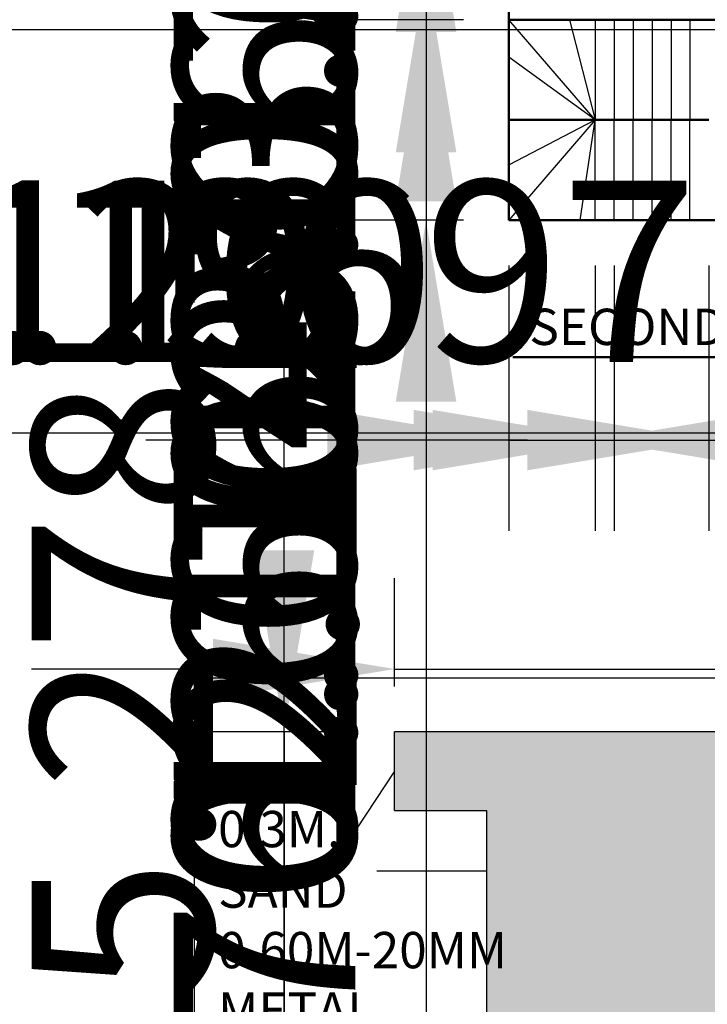
# Model space of a CAD drawing. Units: metres. Extents: x 782 to 1487, y 1262 to 7446.
# Tile 8 of 25: x 821.23 to 830.69, y 1279.51 to 1293.07. Entities that reach past the tile are written whole.
import ezdxf

# ---------------------------------------------------------------- set-up
doc = ezdxf.new("R2010")
doc.units = ezdxf.units.M
for name, color, linetype, lineweight in [('A-ANNO-DIMS', 2, 'Continuous', 18), ('A-ANNO-TEXT', 3, 'Continuous', 18), ('A-DETL', 7, 'Continuous', 25), ('A-DETL-PATT', 9, 'Continuous', 13), ('A-FLOR-STRS', 3, 'Continuous', 25), ('A-WALL', 7, 'Continuous', 50)]:
    doc.layers.add(name, color=color, linetype=linetype, lineweight=lineweight)
doc.styles.get("Standard").update_dxf_attribs({"font": 'arial.ttf'})
doc.dimstyles.new('ISO-25', dxfattribs={"dimtxt": 2.5, "dimasz": 2.5, "dimexe": 1.25, "dimexo": 0.625, "dimtad": 1, "dimtxsty": 'Standard', "dimcen": 2.5, "dimadec": 0, "dimazin": 0, "dimtfac": 1, "dimtmove": 0, "dimatfit": 3, "dimfxl": 1, "dimarcsym": 0})

# ---------------------------------------------------------------- blocks, each defined once
blk = doc.blocks.new('*D10')
at = {"layer": 'A-ANNO-DIMS', "color": 0, "lineweight": -2, "transparency": 16777216}
for p, q in [((825.73, 1277.527), (825.73, 1276.166)), ((826.753, 1277.552), (826.753, 1276.166)), ((823.23, 1277.416), (820.73, 1277.416)), ((825.73, 1277.416), (826.753, 1277.416)), ((829.253, 1277.416), (839.235, 1277.416))]:
    blk.add_line(p, q, dxfattribs=at)
at = {"layer": 'A-ANNO-DIMS', "color": 0, "transparency": 16777216}
for points in [[(823.23, 1277.833), (823.23, 1276.999), (825.73, 1277.416)], [(829.253, 1277.833), (829.253, 1276.999), (826.753, 1277.416)]]:
    blk.add_solid(points, dxfattribs=at)
at = {"layer": 'Defpoints', "color": 0, "transparency": 16777216}
for p in [(826.753, 1278.177), (825.73, 1278.152), (826.753, 1277.416)]:
    blk.add_point(p, dxfattribs=at)
at = {"layer": 'A-ANNO-DIMS', "color": 0, "transparency": 16777216, "insert": (835.494, 1279.543), "char_height": 2.5, "attachment_point": 5}
blk.add_mtext('1,02', dxfattribs=at)
blk = doc.blocks.new('*D22')
at = {"layer": 'A-ANNO-DIMS', "color": 0, "lineweight": -2, "transparency": 16777216}
for p, q in [((812.79, 1292.934), (810.29, 1292.934)), ((815.29, 1292.934), (816.179, 1292.934)), ((818.679, 1292.934), (848.834, 1292.934)), ((815.29, 1292.442), (815.29, 1291.684)), ((816.179, 1292.442), (816.179, 1291.684))]:
    blk.add_line(p, q, dxfattribs=at)
at = {"layer": 'A-ANNO-DIMS', "color": 0, "transparency": 16777216}
for points in [[(812.79, 1293.351), (812.79, 1292.517), (815.29, 1292.934)], [(818.679, 1293.351), (818.679, 1292.517), (816.179, 1292.934)]]:
    blk.add_solid(points, dxfattribs=at)
at = {"layer": 'Defpoints', "color": 0, "transparency": 16777216}
for p in [(815.29, 1293.067), (816.179, 1293.067), (816.179, 1292.934)]:
    blk.add_point(p, dxfattribs=at)
at = {"layer": 'A-ANNO-DIMS', "color": 0, "transparency": 16777216, "insert": (835.007, 1294.852), "char_height": 2.5, "attachment_point": 5}
blk.add_mtext('DOOR 0.89 TYP.', dxfattribs=at)
blk = doc.blocks.new('*D24')
at = {"layer": 'A-ANNO-DIMS', "color": 0, "lineweight": -2, "transparency": 16777216}
for p, q in [((811.209, 1294.423), (808.709, 1294.423)), ((813.709, 1294.423), (814.559, 1294.423)), ((817.059, 1294.423), (852.649, 1294.423)), ((813.709, 1293.926), (813.709, 1293.173)), ((814.559, 1293.926), (814.559, 1293.173))]:
    blk.add_line(p, q, dxfattribs=at)
at = {"layer": 'A-ANNO-DIMS', "color": 0, "transparency": 16777216}
for points in [[(811.209, 1294.84), (811.209, 1294.006), (813.709, 1294.423)], [(817.059, 1294.84), (817.059, 1294.006), (814.559, 1294.423)]]:
    blk.add_solid(points, dxfattribs=at)
at = {"layer": 'Defpoints', "color": 0, "transparency": 16777216}
for p in [(813.709, 1294.551), (814.559, 1294.551), (814.559, 1294.423)]:
    blk.add_point(p, dxfattribs=at)
at = {"layer": 'A-ANNO-DIMS', "color": 0, "transparency": 16777216, "insert": (836.104, 1296.342), "char_height": 2.5, "attachment_point": 5}
blk.add_mtext('DOOR D2 0.85 TYP.', dxfattribs=at)
blk = doc.blocks.new('*D73')
at = {"layer": 'A-ANNO-DIMS', "color": 0, "lineweight": -2, "transparency": 16777216}
for p, q in [((812.13, 1289.68), (812.13, 1286.127)), ((813.319, 1289.68), (813.319, 1286.127)), ((809.63, 1287.377), (807.13, 1287.377)), ((812.13, 1287.377), (813.319, 1287.377)), ((815.819, 1287.377), (825.832, 1287.377))]:
    blk.add_line(p, q, dxfattribs=at)
at = {"layer": 'A-ANNO-DIMS', "color": 0, "transparency": 16777216}
for points in [[(809.63, 1287.794), (809.63, 1286.96), (812.13, 1287.377)], [(815.819, 1287.794), (815.819, 1286.96), (813.319, 1287.377)]]:
    blk.add_solid(points, dxfattribs=at)
at = {"layer": 'Defpoints', "color": 0, "transparency": 16777216}
for p in [(812.13, 1290.305), (813.319, 1290.305), (813.319, 1287.377)]:
    blk.add_point(p, dxfattribs=at)
at = {"layer": 'A-ANNO-DIMS', "color": 0, "transparency": 16777216, "insert": (822.076, 1289.278), "char_height": 2.5, "attachment_point": 5}
blk.add_mtext('1.19', dxfattribs=at)
blk = doc.blocks.new('*D74')
at = {"layer": 'A-ANNO-DIMS', "color": 0, "lineweight": -2, "transparency": 16777216}
for p, q in [((813.319, 1289.68), (813.319, 1286.127)), ((813.58, 1289.68), (813.58, 1286.127)), ((810.819, 1287.377), (808.319, 1287.377)), ((813.319, 1287.377), (813.58, 1287.377)), ((816.08, 1287.377), (826.322, 1287.377))]:
    blk.add_line(p, q, dxfattribs=at)
at = {"layer": 'A-ANNO-DIMS', "color": 0, "transparency": 16777216}
for points in [[(810.819, 1287.794), (810.819, 1286.96), (813.319, 1287.377)], [(816.08, 1287.794), (816.08, 1286.96), (813.58, 1287.377)]]:
    blk.add_solid(points, dxfattribs=at)
at = {"layer": 'Defpoints', "color": 0, "transparency": 16777216}
for p in [(813.319, 1290.305), (813.58, 1290.305), (813.58, 1287.377)]:
    blk.add_point(p, dxfattribs=at)
at = {"layer": 'A-ANNO-DIMS', "color": 0, "transparency": 16777216, "insert": (822.451, 1289.278), "char_height": 2.5, "attachment_point": 5}
blk.add_mtext('0.26', dxfattribs=at)
blk = doc.blocks.new('*D75')
at = {"layer": 'A-ANNO-DIMS', "color": 0, "lineweight": -2, "transparency": 16777216}
for p, q in [((813.58, 1289.68), (813.58, 1286.127)), ((814.883, 1289.68), (814.883, 1286.127)), ((811.08, 1287.377), (808.58, 1287.377)), ((813.58, 1287.377), (814.883, 1287.377)), ((817.383, 1287.377), (827.383, 1287.377))]:
    blk.add_line(p, q, dxfattribs=at)
at = {"layer": 'A-ANNO-DIMS', "color": 0, "transparency": 16777216}
for points in [[(811.08, 1287.794), (811.08, 1286.96), (813.58, 1287.377)], [(817.383, 1287.794), (817.383, 1286.96), (814.883, 1287.377)]]:
    blk.add_solid(points, dxfattribs=at)
at = {"layer": 'Defpoints', "color": 0, "transparency": 16777216}
for p in [(813.58, 1290.305), (814.883, 1290.305), (814.883, 1287.377)]:
    blk.add_point(p, dxfattribs=at)
at = {"layer": 'A-ANNO-DIMS', "color": 0, "transparency": 16777216, "insert": (823.633, 1289.279), "char_height": 2.5, "attachment_point": 5}
blk.add_mtext('1.30', dxfattribs=at)
blk = doc.blocks.new('*D76')
at = {"layer": 'A-ANNO-DIMS', "color": 0, "lineweight": -2, "transparency": 16777216}
for p, q in [((814.883, 1289.68), (814.883, 1286.127)), ((816.58, 1289.68), (816.58, 1286.127)), ((812.383, 1287.377), (809.883, 1287.377)), ((814.883, 1287.377), (816.58, 1287.377)), ((819.08, 1287.377), (831.031, 1287.377))]:
    blk.add_line(p, q, dxfattribs=at)
at = {"layer": 'A-ANNO-DIMS', "color": 0, "transparency": 16777216}
for points in [[(812.383, 1287.794), (812.383, 1286.96), (814.883, 1287.377)], [(819.08, 1287.794), (819.08, 1286.96), (816.58, 1287.377)]]:
    blk.add_solid(points, dxfattribs=at)
at = {"layer": 'Defpoints', "color": 0, "transparency": 16777216}
for p in [(814.883, 1290.305), (816.58, 1290.305), (816.58, 1287.377)]:
    blk.add_point(p, dxfattribs=at)
at = {"layer": 'A-ANNO-DIMS', "color": 0, "transparency": 16777216, "insert": (826.305, 1289.278), "char_height": 2.5, "attachment_point": 5}
blk.add_mtext('1.697', dxfattribs=at)
blk = doc.blocks.new('*D77')
at = {"layer": 'A-ANNO-DIMS', "color": 0, "lineweight": -2, "transparency": 16777216}
for p, q in [((826.821, 1309.827), (826.821, 1312.327)), ((827.337, 1307.327), (825.571, 1307.327)), ((826.821, 1307.327), (826.821, 1304.697)), ((827.567, 1304.697), (825.571, 1304.697)), ((826.821, 1302.197), (826.821, 1291.911))]:
    blk.add_line(p, q, dxfattribs=at)
at = {"layer": 'A-ANNO-DIMS', "color": 0, "transparency": 16777216}
for points in [[(826.404, 1309.827), (827.238, 1309.827), (826.821, 1307.327)], [(826.404, 1302.197), (827.238, 1302.197), (826.821, 1304.697)]]:
    blk.add_solid(points, dxfattribs=at)
at = {"layer": 'Defpoints', "color": 0, "transparency": 16777216}
for p in [(827.962, 1307.327), (826.821, 1304.697), (828.192, 1304.697)]:
    blk.add_point(p, dxfattribs=at)
at = {"layer": 'A-ANNO-DIMS', "color": 0, "transparency": 16777216, "insert": (824.919, 1295.804), "char_height": 2.5, "attachment_point": 5, "rotation": 90}
blk.add_mtext('2.63', dxfattribs=at)
blk = doc.blocks.new('*D78')
at = {"layer": 'A-ANNO-DIMS', "color": 0, "lineweight": -2, "transparency": 16777216}
for p, q in [((826.821, 1307.197), (826.821, 1309.697)), ((827.567, 1304.697), (825.571, 1304.697)), ((826.821, 1304.697), (826.821, 1302.822)), ((827.336, 1302.822), (825.571, 1302.822)), ((826.821, 1300.322), (826.821, 1290.308))]:
    blk.add_line(p, q, dxfattribs=at)
at = {"layer": 'A-ANNO-DIMS', "color": 0, "transparency": 16777216}
for points in [[(826.404, 1307.197), (827.238, 1307.197), (826.821, 1304.697)], [(826.404, 1300.322), (827.238, 1300.322), (826.821, 1302.822)]]:
    blk.add_solid(points, dxfattribs=at)
at = {"layer": 'Defpoints', "color": 0, "transparency": 16777216}
for p in [(828.192, 1304.697), (826.821, 1302.822), (827.961, 1302.822)]:
    blk.add_point(p, dxfattribs=at)
at = {"layer": 'A-ANNO-DIMS', "color": 0, "transparency": 16777216, "insert": (824.919, 1294.065), "char_height": 2.5, "attachment_point": 5, "rotation": 90}
blk.add_mtext('1.88', dxfattribs=at)
blk = doc.blocks.new('*D79')
at = {"layer": 'A-ANNO-DIMS', "color": 0, "lineweight": -2, "transparency": 16777216}
for p, q in [((826.821, 1305.322), (826.821, 1307.822)), ((827.336, 1302.822), (825.571, 1302.822)), ((826.821, 1302.822), (826.821, 1302.177)), ((827.567, 1302.177), (825.571, 1302.177)), ((826.821, 1299.677), (826.821, 1289.444))]:
    blk.add_line(p, q, dxfattribs=at)
at = {"layer": 'A-ANNO-DIMS', "color": 0, "transparency": 16777216}
for points in [[(826.404, 1305.322), (827.238, 1305.322), (826.821, 1302.822)], [(826.404, 1299.677), (827.238, 1299.677), (826.821, 1302.177)]]:
    blk.add_solid(points, dxfattribs=at)
at = {"layer": 'Defpoints', "color": 0, "transparency": 16777216}
for p in [(827.961, 1302.822), (826.821, 1302.177), (828.192, 1302.177)]:
    blk.add_point(p, dxfattribs=at)
at = {"layer": 'A-ANNO-DIMS', "color": 0, "transparency": 16777216, "insert": (824.919, 1293.311), "char_height": 2.5, "attachment_point": 5, "rotation": 90}
blk.add_mtext('0.64', dxfattribs=at)
blk = doc.blocks.new('*D80')
at = {"layer": 'A-ANNO-DIMS', "color": 0, "lineweight": -2, "transparency": 16777216}
for p, q in [((826.821, 1304.677), (826.821, 1307.177)), ((827.567, 1302.177), (825.571, 1302.177)), ((826.821, 1302.177), (826.821, 1299.809)), ((827.338, 1299.809), (825.571, 1299.809)), ((826.821, 1297.309), (826.821, 1287.022))]:
    blk.add_line(p, q, dxfattribs=at)
at = {"layer": 'A-ANNO-DIMS', "color": 0, "transparency": 16777216}
for points in [[(826.404, 1304.677), (827.238, 1304.677), (826.821, 1302.177)], [(826.404, 1297.309), (827.238, 1297.309), (826.821, 1299.809)]]:
    blk.add_solid(points, dxfattribs=at)
at = {"layer": 'Defpoints', "color": 0, "transparency": 16777216}
for p in [(828.192, 1302.177), (826.821, 1299.809), (827.963, 1299.809)]:
    blk.add_point(p, dxfattribs=at)
at = {"layer": 'A-ANNO-DIMS', "color": 0, "transparency": 16777216, "insert": (824.919, 1290.916), "char_height": 2.5, "attachment_point": 5, "rotation": 90}
blk.add_mtext('2.37', dxfattribs=at)
blk = doc.blocks.new('*D81')
at = {"layer": 'A-ANNO-DIMS', "color": 0, "lineweight": -2, "transparency": 16777216}
for p, q in [((826.821, 1302.309), (826.821, 1304.809)), ((827.338, 1299.809), (825.571, 1299.809)), ((826.821, 1299.809), (826.821, 1298.647)), ((827.567, 1298.647), (825.571, 1298.647)), ((826.821, 1296.147), (826.821, 1286.141))]:
    blk.add_line(p, q, dxfattribs=at)
at = {"layer": 'A-ANNO-DIMS', "color": 0, "transparency": 16777216}
for points in [[(826.404, 1302.309), (827.238, 1302.309), (826.821, 1299.809)], [(826.404, 1296.147), (827.238, 1296.147), (826.821, 1298.647)]]:
    blk.add_solid(points, dxfattribs=at)
at = {"layer": 'Defpoints', "color": 0, "transparency": 16777216}
for p in [(827.963, 1299.809), (826.821, 1298.647), (828.192, 1298.647)]:
    blk.add_point(p, dxfattribs=at)
at = {"layer": 'A-ANNO-DIMS', "color": 0, "transparency": 16777216, "insert": (824.919, 1289.894), "char_height": 2.5, "attachment_point": 5, "rotation": 90}
blk.add_mtext('1.16', dxfattribs=at)
blk = doc.blocks.new('*D82')
at = {"layer": 'A-ANNO-DIMS', "color": 0, "lineweight": -2, "transparency": 16777216}
for p, q in [((826.821, 1301.147), (826.821, 1303.647)), ((827.567, 1298.647), (825.571, 1298.647)), ((826.821, 1298.647), (826.821, 1296.5)), ((827.339, 1296.5), (825.571, 1296.5)), ((826.821, 1294), (826.821, 1281.772))]:
    blk.add_line(p, q, dxfattribs=at)
at = {"layer": 'A-ANNO-DIMS', "color": 0, "transparency": 16777216}
for points in [[(826.404, 1301.147), (827.238, 1301.147), (826.821, 1298.647)], [(826.404, 1294), (827.238, 1294), (826.821, 1296.5)]]:
    blk.add_solid(points, dxfattribs=at)
at = {"layer": 'Defpoints', "color": 0, "transparency": 16777216}
for p in [(828.192, 1298.647), (826.821, 1296.5), (827.964, 1296.5)]:
    blk.add_point(p, dxfattribs=at)
at = {"layer": 'A-ANNO-DIMS', "color": 0, "transparency": 16777216, "insert": (824.941, 1286.636), "char_height": 2.5, "attachment_point": 5, "rotation": 90}
blk.add_mtext('2.147', dxfattribs=at)
blk = doc.blocks.new('*D83')
at = {"layer": 'A-ANNO-DIMS', "color": 0, "lineweight": -2, "transparency": 16777216}
for p, q in [((826.821, 1299), (826.821, 1301.5)), ((827.339, 1296.5), (825.571, 1296.5)), ((826.821, 1296.5), (826.821, 1295.397)), ((827.567, 1295.397), (825.571, 1295.397)), ((826.821, 1292.897), (826.821, 1280.947))]:
    blk.add_line(p, q, dxfattribs=at)
at = {"layer": 'A-ANNO-DIMS', "color": 0, "transparency": 16777216}
for points in [[(826.404, 1299), (827.238, 1299), (826.821, 1296.5)], [(826.404, 1292.897), (827.238, 1292.897), (826.821, 1295.397)]]:
    blk.add_solid(points, dxfattribs=at)
at = {"layer": 'Defpoints', "color": 0, "transparency": 16777216}
for p in [(827.964, 1296.5), (826.821, 1295.397), (828.192, 1295.397)]:
    blk.add_point(p, dxfattribs=at)
at = {"layer": 'A-ANNO-DIMS', "color": 0, "transparency": 16777216, "insert": (824.919, 1285.672), "char_height": 2.5, "attachment_point": 5, "rotation": 90}
blk.add_mtext('1.103', dxfattribs=at)
blk = doc.blocks.new('*D84')
at = {"layer": 'A-ANNO-DIMS', "color": 0, "lineweight": -2, "transparency": 16777216}
for p, q in [((826.821, 1297.897), (826.821, 1300.397)), ((827.567, 1295.397), (825.571, 1295.397)), ((826.821, 1295.397), (826.821, 1293.74)), ((827.337, 1293.74), (825.571, 1293.74)), ((826.821, 1291.24), (826.821, 1281.233))]:
    blk.add_line(p, q, dxfattribs=at)
at = {"layer": 'A-ANNO-DIMS', "color": 0, "transparency": 16777216}
for points in [[(826.404, 1297.897), (827.238, 1297.897), (826.821, 1295.397)], [(826.404, 1291.24), (827.238, 1291.24), (826.821, 1293.74)]]:
    blk.add_solid(points, dxfattribs=at)
at = {"layer": 'Defpoints', "color": 0, "transparency": 16777216}
for p in [(828.192, 1295.397), (826.821, 1293.74), (827.962, 1293.74)]:
    blk.add_point(p, dxfattribs=at)
at = {"layer": 'A-ANNO-DIMS', "color": 0, "transparency": 16777216, "insert": (824.919, 1284.987), "char_height": 2.5, "attachment_point": 5, "rotation": 90}
blk.add_mtext('1.66', dxfattribs=at)
blk = doc.blocks.new('*D85')
at = {"layer": 'A-ANNO-DIMS', "color": 0, "lineweight": -2, "transparency": 16777216}
for p, q in [((826.821, 1296.24), (826.821, 1298.74)), ((827.337, 1293.74), (825.571, 1293.74)), ((826.821, 1293.74), (826.821, 1293.067)), ((827.337, 1293.067), (825.571, 1293.067)), ((826.821, 1290.567), (826.821, 1280.324))]:
    blk.add_line(p, q, dxfattribs=at)
at = {"layer": 'A-ANNO-DIMS', "color": 0, "transparency": 16777216}
for points in [[(826.404, 1296.24), (827.238, 1296.24), (826.821, 1293.74)], [(826.404, 1290.567), (827.238, 1290.567), (826.821, 1293.067)]]:
    blk.add_solid(points, dxfattribs=at)
at = {"layer": 'Defpoints', "color": 0, "transparency": 16777216}
for p in [(827.962, 1293.74), (826.821, 1293.067), (827.962, 1293.067)]:
    blk.add_point(p, dxfattribs=at)
at = {"layer": 'A-ANNO-DIMS', "color": 0, "transparency": 16777216, "insert": (824.919, 1284.195), "char_height": 2.5, "attachment_point": 5, "rotation": 90}
blk.add_mtext('0.67', dxfattribs=at)
blk = doc.blocks.new('*D86')
at = {"layer": 'A-ANNO-DIMS', "color": 0, "lineweight": -2, "transparency": 16777216}
for p, q in [((826.821, 1295.567), (826.821, 1298.067)), ((827.337, 1293.067), (825.571, 1293.067)), ((826.821, 1293.067), (826.821, 1290.305)), ((827.337, 1290.305), (825.571, 1290.305)), ((826.821, 1287.805), (826.821, 1275.602))]:
    blk.add_line(p, q, dxfattribs=at)
at = {"layer": 'A-ANNO-DIMS', "color": 0, "transparency": 16777216}
for points in [[(826.404, 1295.567), (827.238, 1295.567), (826.821, 1293.067)], [(826.404, 1287.805), (827.238, 1287.805), (826.821, 1290.305)]]:
    blk.add_solid(points, dxfattribs=at)
at = {"layer": 'Defpoints', "color": 0, "transparency": 16777216}
for p in [(827.962, 1293.067), (826.821, 1290.305), (827.962, 1290.305)]:
    blk.add_point(p, dxfattribs=at)
at = {"layer": 'A-ANNO-DIMS', "color": 0, "transparency": 16777216, "insert": (824.919, 1280.454), "char_height": 2.5, "attachment_point": 5, "rotation": 90}
blk.add_mtext('2.762', dxfattribs=at)
blk = doc.blocks.new('*D97')
at = {"layer": 'A-ANNO-DIMS', "color": 0, "lineweight": -2, "transparency": 16777216}
for p, q in [((827.962, 1289.68), (827.962, 1286.027)), ((829.151, 1289.68), (829.151, 1286.027)), ((825.462, 1287.277), (822.962, 1287.277)), ((827.962, 1287.277), (829.151, 1287.277)), ((831.651, 1287.277), (841.665, 1287.277))]:
    blk.add_line(p, q, dxfattribs=at)
at = {"layer": 'A-ANNO-DIMS', "color": 0, "transparency": 16777216}
for points in [[(825.462, 1287.694), (825.462, 1286.861), (827.962, 1287.277)], [(831.651, 1287.694), (831.651, 1286.861), (829.151, 1287.277)]]:
    blk.add_solid(points, dxfattribs=at)
at = {"layer": 'Defpoints', "color": 0, "transparency": 16777216}
for p in [(827.962, 1290.305), (829.151, 1290.305), (829.151, 1287.277)]:
    blk.add_point(p, dxfattribs=at)
at = {"layer": 'A-ANNO-DIMS', "color": 0, "transparency": 16777216, "insert": (837.908, 1289.179), "char_height": 2.5, "attachment_point": 5}
blk.add_mtext('1.19', dxfattribs=at)
blk = doc.blocks.new('*D98')
at = {"layer": 'A-ANNO-DIMS', "color": 0, "lineweight": -2, "transparency": 16777216}
for p, q in [((829.151, 1289.68), (829.151, 1286.027)), ((829.412, 1289.68), (829.412, 1286.027)), ((826.651, 1287.277), (824.151, 1287.277)), ((829.151, 1287.277), (829.412, 1287.277)), ((831.912, 1287.277), (842.154, 1287.277))]:
    blk.add_line(p, q, dxfattribs=at)
at = {"layer": 'A-ANNO-DIMS', "color": 0, "transparency": 16777216}
for points in [[(826.651, 1287.694), (826.651, 1286.861), (829.151, 1287.277)], [(831.912, 1287.694), (831.912, 1286.861), (829.412, 1287.277)]]:
    blk.add_solid(points, dxfattribs=at)
at = {"layer": 'Defpoints', "color": 0, "transparency": 16777216}
for p in [(829.151, 1290.305), (829.412, 1290.305), (829.412, 1287.277)]:
    blk.add_point(p, dxfattribs=at)
at = {"layer": 'A-ANNO-DIMS', "color": 0, "transparency": 16777216, "insert": (838.283, 1289.179), "char_height": 2.5, "attachment_point": 5}
blk.add_mtext('0.26', dxfattribs=at)
blk = doc.blocks.new('*D99')
at = {"layer": 'A-ANNO-DIMS', "color": 0, "lineweight": -2, "transparency": 16777216}
for p, q in [((829.412, 1289.68), (829.412, 1286.027)), ((830.716, 1289.68), (830.716, 1286.027)), ((826.912, 1287.277), (824.412, 1287.277)), ((829.412, 1287.277), (830.716, 1287.277)), ((833.216, 1287.277), (843.216, 1287.277))]:
    blk.add_line(p, q, dxfattribs=at)
at = {"layer": 'A-ANNO-DIMS', "color": 0, "transparency": 16777216}
for points in [[(826.912, 1287.694), (826.912, 1286.861), (829.412, 1287.277)], [(833.216, 1287.694), (833.216, 1286.861), (830.716, 1287.277)]]:
    blk.add_solid(points, dxfattribs=at)
at = {"layer": 'Defpoints', "color": 0, "transparency": 16777216}
for p in [(829.412, 1290.305), (830.716, 1290.305), (830.716, 1287.277)]:
    blk.add_point(p, dxfattribs=at)
at = {"layer": 'A-ANNO-DIMS', "color": 0, "transparency": 16777216, "insert": (839.466, 1289.18), "char_height": 2.5, "attachment_point": 5}
blk.add_mtext('1.30', dxfattribs=at)
blk = doc.blocks.new('*D100')
at = {"layer": 'A-ANNO-DIMS', "color": 0, "lineweight": -2, "transparency": 16777216}
for p, q in [((830.716, 1289.68), (830.716, 1286.027)), ((832.412, 1289.68), (832.412, 1286.027)), ((828.216, 1287.277), (825.716, 1287.277)), ((830.716, 1287.277), (832.412, 1287.277)), ((834.912, 1287.277), (846.863, 1287.277))]:
    blk.add_line(p, q, dxfattribs=at)
at = {"layer": 'A-ANNO-DIMS', "color": 0, "transparency": 16777216}
for points in [[(828.216, 1287.694), (828.216, 1286.861), (830.716, 1287.277)], [(834.912, 1287.694), (834.912, 1286.861), (832.412, 1287.277)]]:
    blk.add_solid(points, dxfattribs=at)
at = {"layer": 'Defpoints', "color": 0, "transparency": 16777216}
for p in [(830.716, 1290.305), (832.412, 1290.305), (832.412, 1287.277)]:
    blk.add_point(p, dxfattribs=at)
at = {"layer": 'A-ANNO-DIMS', "color": 0, "transparency": 16777216, "insert": (842.138, 1289.179), "char_height": 2.5, "attachment_point": 5}
blk.add_mtext('1.697', dxfattribs=at)
blk = doc.blocks.new('*D163')
at = {"layer": 'A-ANNO-DIMS', "color": 0, "lineweight": -2, "transparency": 16777216}
for p, q in [((824.865, 1276.532), (824.865, 1288.723)), ((826.79, 1274.032), (823.615, 1274.032)), ((824.865, 1268.754), (824.865, 1274.032)), ((826.79, 1268.754), (823.615, 1268.754)), ((824.865, 1266.254), (824.865, 1263.754))]:
    blk.add_line(p, q, dxfattribs=at)
at = {"layer": 'A-ANNO-DIMS', "color": 0, "transparency": 16777216}
for points in [[(824.448, 1276.532), (825.281, 1276.532), (824.865, 1274.032)], [(824.448, 1266.254), (825.281, 1266.254), (824.865, 1268.754)]]:
    blk.add_solid(points, dxfattribs=at)
at = {"layer": 'Defpoints', "color": 0, "transparency": 16777216}
for p in [(824.865, 1274.032), (827.415, 1274.032), (827.415, 1268.754)]:
    blk.add_point(p, dxfattribs=at)
at = {"layer": 'A-ANNO-DIMS', "color": 0, "transparency": 16777216, "insert": (822.963, 1283.878), "char_height": 2.5, "attachment_point": 5, "rotation": 90}
blk.add_mtext('5.278', dxfattribs=at)
blk = doc.blocks.new('*D165')
at = {"layer": 'A-ANNO-DIMS', "color": 0, "lineweight": -2, "transparency": 16777216}
for p, q in [((826.388, 1283.885), (826.388, 1285.375)), ((832.011, 1283.885), (832.011, 1285.375)), ((823.888, 1284.125), (821.388, 1284.125)), ((826.388, 1284.125), (832.011, 1284.125)), ((834.511, 1284.125), (846.697, 1284.125))]:
    blk.add_line(p, q, dxfattribs=at)
at = {"layer": 'A-ANNO-DIMS', "color": 0, "transparency": 16777216}
for points in [[(823.888, 1284.541), (823.888, 1283.708), (826.388, 1284.125)], [(834.511, 1284.541), (834.511, 1283.708), (832.011, 1284.125)]]:
    blk.add_solid(points, dxfattribs=at)
at = {"layer": 'Defpoints', "color": 0, "transparency": 16777216}
for p in [(832.011, 1284.125), (826.388, 1283.26), (832.011, 1283.26)]:
    blk.add_point(p, dxfattribs=at)
at = {"layer": 'A-ANNO-DIMS', "color": 0, "transparency": 16777216, "insert": (841.854, 1286.027), "char_height": 2.5, "attachment_point": 5}
blk.add_mtext('5.623', dxfattribs=at)
blk = doc.blocks.new('*D166')
at = {"layer": 'A-ANNO-DIMS', "color": 0, "lineweight": -2, "transparency": 16777216}
for p, q in [((824.865, 1285.76), (824.865, 1288.26)), ((825.763, 1283.26), (823.615, 1283.26)), ((824.865, 1283.26), (824.865, 1279.121)), ((827.029, 1279.121), (823.615, 1279.121)), ((824.865, 1276.621), (824.865, 1264.329))]:
    blk.add_line(p, q, dxfattribs=at)
at = {"layer": 'A-ANNO-DIMS', "color": 0, "transparency": 16777216}
for points in [[(824.448, 1285.76), (825.281, 1285.76), (824.865, 1283.26)], [(824.448, 1276.621), (825.281, 1276.621), (824.865, 1279.121)]]:
    blk.add_solid(points, dxfattribs=at)
at = {"layer": 'Defpoints', "color": 0, "transparency": 16777216}
for p in [(826.388, 1283.26), (824.865, 1279.121), (827.654, 1279.121)]:
    blk.add_point(p, dxfattribs=at)
at = {"layer": 'A-ANNO-DIMS', "color": 0, "transparency": 16777216, "insert": (822.962, 1269.225), "char_height": 2.5, "attachment_point": 5, "rotation": 90}
blk.add_mtext('4.138', dxfattribs=at)

msp = doc.modelspace()

# ---------------------------------------------------------------- hatches: boundary and pattern name
at = {"layer": 'A-DETL-PATT'}
h = msp.add_hatch(color=256, dxfattribs=at)
h.dxf.hatch_style = 1
h.paths.add_polyline_path([(831.1207, 1282.1784), (832.0105, 1282.1784), (832.0105, 1283.2597), (826.3877, 1283.2597), (826.3877, 1282.1784), (827.6538, 1282.1784), (827.6538, 1279.1214), (831.1207, 1279.1214)])
h.paths.add_polyline_path([(823.78, 1277.2166), (828.1675, 1277.2166), (828.1675, 1282.4262), (823.78, 1282.4262)], flags=9)
h = msp.add_hatch(color=256, dxfattribs=at)
h.dxf.hatch_style = 1
h.paths.add_polyline_path([(831.1207, 1282.1784), (832.0105, 1282.1784), (832.0105, 1283.2597), (826.3877, 1283.2597), (826.3877, 1282.1784), (827.6538, 1282.1784), (827.6538, 1279.1214), (831.1207, 1279.1214)])
h.paths.add_polyline_path([(823.78, 1277.2166), (828.1675, 1277.2166), (828.1675, 1282.4262), (823.78, 1282.4262)], flags=9)

# ---------------------------------------------------------------- linework, layer by layer
at = {"layer": 'A-DETL'}
for p, q in [((832.0105, 1283.2597), (826.3877, 1283.2597)), ((826.3877, 1282.1784), (826.3877, 1283.2597)), ((826.3877, 1282.7191), (825.7296, 1281.7233)), ((826.3877, 1282.1784), (827.6538, 1282.1784)), ((827.6538, 1282.1784), (827.6538, 1279.1214)), ((826.1411, 1281.3437), (826.7525, 1281.3437)), ((826.7525, 1281.3437), (827.6538, 1281.3437))]:
    msp.add_line(p, q, dxfattribs=at)
msp.add_lwpolyline([(823.6278, 1284.0012), (823.6278, 1266.59), (847.1334, 1266.59), (847.1334, 1284.0012)], close=True, dxfattribs=at)
at = {"layer": 'A-FLOR-STRS'}
for p, q in [((829.1513, 1291.6863), (827.9625, 1293.0674)), ((829.1513, 1293.0674), (828.7975, 1293.0674)), ((828.7975, 1293.0674), (829.1513, 1291.6863)), ((829.1513, 1293.0674), (829.1513, 1291.6863)), ((829.412, 1293.0674), (829.412, 1291.6863)), ((829.6727, 1293.0674), (829.6727, 1291.6863)), ((829.9335, 1293.0674), (829.9335, 1291.6863)), ((830.1942, 1293.0674), (830.1942, 1291.6863)), ((830.4549, 1293.0674), (830.4549, 1291.6863)), ((829.1513, 1291.6863), (827.9625, 1292.5526)), ((829.1513, 1291.6863), (827.9625, 1290.3053)), ((829.1513, 1291.6863), (827.9625, 1291.6863)), ((827.9625, 1291.0666), (829.1513, 1291.6863)), ((828.9433, 1290.3053), (829.1513, 1291.6863)), ((829.1513, 1290.3053), (829.1513, 1291.6863)), ((829.412, 1290.3053), (829.412, 1291.6863)), ((829.6727, 1290.3053), (829.6727, 1291.6863)), ((829.9335, 1290.3053), (829.9335, 1291.6863)), ((830.1942, 1290.3053), (830.1942, 1291.6863)), ((830.4549, 1290.3053), (830.4549, 1291.6863))]:
    msp.add_line(p, q, dxfattribs=at)
at = {"layer": 'A-WALL'}
for p, q in [((827.9625, 1295.3974), (827.9625, 1293.0674)), ((827.9625, 1293.0674), (830.6725, 1293.0674)), ((827.9625, 1293.0674), (827.9625, 1290.3053)), ((832.4125, 1293.0674), (827.9625, 1293.0674)), ((830.6725, 1293.0674), (831.1618, 1293.0674)), ((830.7156, 1291.6863), (827.9625, 1291.6863)), ((830.7156, 1291.6863), (827.9625, 1291.6863)), ((827.9625, 1291.6863), (827.9625, 1291.0666)), ((827.9625, 1290.3053), (832.4125, 1290.3053)), ((827.9625, 1290.3053), (828.9433, 1290.3053)), ((828.0178, 1288.4175), (834.0505, 1288.4175))]:
    msp.add_line(p, q, dxfattribs=at)

# ---------------------------------------------------------------- texts
at = {"layer": 'A-ANNO-TEXT', "char_height": 0.5, "attachment_point": 1}
for s, width, insert in [('\\PSECONDFLOOR', 4.240641, (828.2435, 1289.921)), ('\\P0.3M. SAND\\P0.60M-20MM METAL\\P0.60M-MM METAL ', 2.795673, (823.9569, 1283.0043))]:
    msp.add_mtext_dynamic_manual_height_columns(s, width=width, gutter_width=12.5, heights=[0], dxfattribs=dict(at, insert=insert))

# ---------------------------------------------------------------- dimensions: what is measured, and where the dimension line sits
at = {"layer": 'A-ANNO-DIMS'}
for base, p1, p2, override, picture, middle in [((826.8209, 1304.6974), (827.9625, 1307.3274), (828.1925, 1304.6974), {"dimdec": 2, "dimlfac": 1, "dimrnd": 0, "dimzin": 0, "dimdsep": 46, "dimlunit": 2}, '*D77', (824.9186, 1295.8042)), ((826.8209, 1302.8221), (828.1925, 1304.6974), (827.9609, 1302.8221), {"dimdec": 2, "dimlfac": 1, "dimrnd": 0, "dimzin": 0, "dimdsep": 46, "dimlunit": 2}, '*D78', (824.9195, 1294.0652)), ((826.8209, 1302.1774), (827.9609, 1302.8221), (828.1925, 1302.1774), {"dimdec": 2, "dimlfac": 1, "dimrnd": 0, "dimzin": 0, "dimdsep": 46, "dimlunit": 2}, '*D79', (824.9195, 1293.3106)), ((826.8209, 1299.8088), (828.1925, 1302.1774), (827.9631, 1299.8088), {"dimdec": 2, "dimlfac": 1, "dimrnd": 0, "dimzin": 0, "dimdsep": 46, "dimlunit": 2}, '*D80', (824.9186, 1290.9156)), ((826.8209, 1298.6474), (827.9631, 1299.8088), (828.1925, 1298.6474), {"dimdec": 2, "dimlfac": 1, "dimrnd": 0, "dimzin": 0, "dimdsep": 46, "dimlunit": 2}, '*D81', (824.9195, 1289.894)), ((826.8209, 1296.5004), (828.1925, 1298.6474), (827.9641, 1296.5004), {"dimdec": 3, "dimlfac": 1, "dimrnd": 0, "dimzin": 0, "dimdsep": 46, "dimlunit": 2}, '*D82', (824.9408, 1286.636)), ((826.8209, 1295.3974), (827.9641, 1296.5004), (828.1925, 1295.3974), {"dimdec": 3, "dimlfac": 1, "dimrnd": 0, "dimzin": 0, "dimdsep": 46, "dimlunit": 2}, '*D83', (824.9186, 1285.672)), ((826.8209, 1293.7402), (828.1925, 1295.3974), (827.9622, 1293.7402), {"dimdec": 2, "dimlfac": 1, "dimrnd": 0, "dimzin": 0, "dimdsep": 46, "dimlunit": 2}, '*D84', (824.9195, 1284.9868)), ((826.8209, 1293.0674), (827.9622, 1293.7402), (827.9625, 1293.0674), {"dimdec": 2, "dimlfac": 1, "dimrnd": 0, "dimzin": 0, "dimdsep": 46, "dimlunit": 2}, '*D85', (824.9195, 1284.1955)), ((826.8209, 1290.3053), (827.9625, 1293.0674), (827.9625, 1290.3053), {"dimdec": 3, "dimlfac": 1, "dimrnd": 0, "dimzin": 0, "dimdsep": 46, "dimlunit": 2}, '*D86', (824.9195, 1280.4536)), ((824.8646, 1274.0318), (827.4151, 1268.754), (827.4151, 1274.0318), {"dimdec": 3, "dimlfac": 1, "dimrnd": 0, "dimzin": 0, "dimdsep": 46, "dimlunit": 2}, '*D163', (822.9632, 1283.8775)), ((824.8646, 1279.1214), (826.3877, 1283.2597), (827.6538, 1279.1214), {"dimdec": 3, "dimlfac": 1, "dimrnd": 0, "dimzin": 0, "dimdsep": 46, "dimlunit": 2}, '*D166', (822.9623, 1269.2254))]:
    dim = msp.add_linear_dim(base=base, p1=p1, p2=p2, angle=90, dimstyle='ISO-25', override=override, dxfattribs=at)
    dim.commit()
    dim.dimension.update_dxf_attribs({"geometry": picture, "text_midpoint": middle})
for base, p1, p2, text, picture, middle in [((814.5592, 1294.4231), (813.7086, 1294.5507), (814.5592, 1294.5507), 'DOOR D2 <> TYP.', '*D24', (836.1042, 1296.3416)), ((816.1792, 1292.934), (815.2897, 1293.0674), (816.1792, 1293.0674), 'DOOR <> TYP.', '*D22', (835.0068, 1294.8525))]:
    dim = msp.add_linear_dim(base=base, p1=p1, p2=p2, text=text, dimstyle='ISO-25', override={"dimdec": 2, "dimlfac": 1, "dimrnd": 0, "dimzin": 0, "dimdsep": 46, "dimlunit": 2}, dxfattribs=at)
    dim.commit()
    dim.dimension.update_dxf_attribs({"geometry": picture, "text_midpoint": middle})
for base, p1, p2, override, picture, middle in [((813.3188, 1287.377), (812.13, 1290.3053), (813.3188, 1290.3053), {"dimdec": 2, "dimlfac": 1, "dimrnd": 0, "dimzin": 0, "dimdsep": 46, "dimlunit": 2}, '*D73', (822.0757, 1289.2784)), ((813.5796, 1287.377), (813.3188, 1290.3053), (813.5796, 1290.3053), {"dimdec": 2, "dimlfac": 1, "dimrnd": 0, "dimzin": 0, "dimdsep": 46, "dimlunit": 2}, '*D74', (822.4506, 1289.2784)), ((814.8832, 1287.377), (813.5796, 1290.3053), (814.8832, 1290.3053), {"dimdec": 2, "dimlfac": 1, "dimrnd": 0, "dimzin": 0, "dimdsep": 46, "dimlunit": 2}, '*D75', (823.6332, 1289.2792)), ((816.58, 1287.377), (814.8832, 1290.3053), (816.58, 1290.3053), {"dimdec": 3, "dimlfac": 1, "dimrnd": 0, "dimzin": 0, "dimdsep": 46, "dimlunit": 2}, '*D76', (826.3055, 1289.2784)), ((829.1513, 1287.2775), (827.9625, 1290.3053), (829.1513, 1290.3053), {"dimdec": 2, "dimlfac": 1, "dimrnd": 0, "dimzin": 0, "dimdsep": 46, "dimlunit": 2}, '*D97', (837.9081, 1289.1789)), ((829.412, 1287.2775), (829.1513, 1290.3053), (829.412, 1290.3053), {"dimdec": 2, "dimlfac": 1, "dimrnd": 0, "dimzin": 0, "dimdsep": 46, "dimlunit": 2}, '*D98', (838.2831, 1289.1789)), ((830.7156, 1287.2775), (829.412, 1290.3053), (830.7156, 1290.3053), {"dimdec": 2, "dimlfac": 1, "dimrnd": 0, "dimzin": 0, "dimdsep": 46, "dimlunit": 2}, '*D99', (839.4656, 1289.1798)), ((832.4125, 1287.2775), (830.7156, 1290.3053), (832.4125, 1290.3053), {"dimdec": 3, "dimlfac": 1, "dimrnd": 0, "dimzin": 0, "dimdsep": 46, "dimlunit": 2}, '*D100', (842.1379, 1289.1789)), ((832.0105, 1284.1247), (826.3877, 1283.2597), (832.0105, 1283.2597), {"dimdec": 3, "dimlfac": 1, "dimrnd": 0, "dimzin": 0, "dimdsep": 46, "dimlunit": 2}, '*D165', (841.8536, 1286.027))]:
    dim = msp.add_linear_dim(base=base, p1=p1, p2=p2, dimstyle='ISO-25', override=override, dxfattribs=at)
    dim.commit()
    dim.dimension.update_dxf_attribs({"geometry": picture, "text_midpoint": middle})
dim = msp.add_linear_dim(base=(826.7525, 1277.4159), p1=(825.7296, 1278.1516), p2=(826.7525, 1278.177), dimstyle='ISO-25', override={"dimclrd": 0, "dimclre": 0, "dimclrt": 0}, dxfattribs=at)
dim.commit()
dim.dimension.update_dxf_attribs({"geometry": '*D10', "text_midpoint": (835.494, 1277.4159), "dimtype": 160})

doc.saveas('drawing.dxf')
